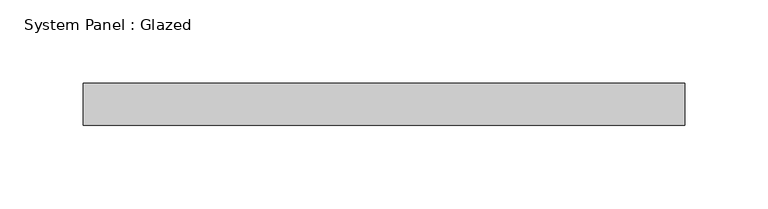
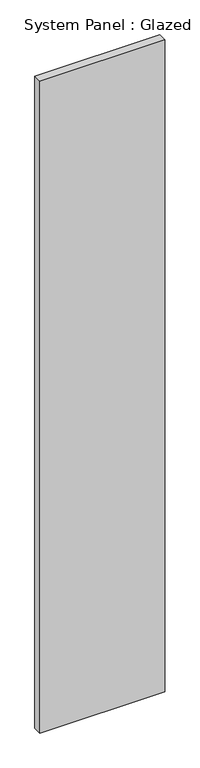
"""IFC4 building model written with IfcOpenShell, lengths in millimetres: plate geometry, System Panel : Glazed."""

from ifc_helpers import new_model, si_unit, origin, origin_with_axes, place, context, project, spatial, polyline, outline, extrude, source, transform, mapped, element, save


def system_panel_glazed_7d1c9128(model_context):
    return source(origin(), model_context, "Body", "SweptSolid", [
        extrude(outline(polyline([(181.3019779, 19.05), (-181.3019779, 19.05), (-181.3019779, 44.45), (181.3019779, 44.45), (181.3019779, 19.05)])), origin_with_axes(), (0.0, 0.0, 1.0), 2001.2825),
    ])


if __name__ == "__main__":
    model = new_model("IFC4")
    model_context = context("Model", 3, world=origin())
    ifc_project = project(units=[si_unit("LENGTHUNIT", "METRE", prefix="MILLI")], contexts=[model_context])
    site = spatial("IfcSite", under=ifc_project)
    building = spatial("IfcBuilding", under=site)
    placement = place(None, origin())
    system_panel_glazed_shape = system_panel_glazed_7d1c9128(model_context)
    element("IfcPlate", 1, ObjectType="System Panel : Glazed", at=placement, inside=building, context=model_context, shape_type="MappedRepresentation", body=[
        mapped(system_panel_glazed_shape, transform((0.0, 0.0, 0.0), x_axis=(1.0, 0.0, 0.0), y_axis=(0.0, 1.0, 0.0), z_axis=(0.0, 0.0, 1.0))),
    ])
    save(model, "model.ifc")

# Revit data of these elements
# Type "System Panel : Glazed"
#   Construction Type Id = "GSP4R"
#   Analytic Construction = "1/8 in Pilkington single glazing"
#   Visual Light Transmittance = 0.9
#   Solar Heat Gain Coefficient = 0.86
#   Heat Transfer Coefficient (U) = 1.18115 BTU/(h·ft²·°F)
#   Define Thermal Properties by = 1
# Element 1 (IfcPlate, "System Panel : Glazed")
#   Materials on its faces: "Glass"
# Materials
#   "Glass": class "Glass", colour RGB 154 182 205, transparency 0.85, Description = "Soda Lime Glass", Cost = 0
